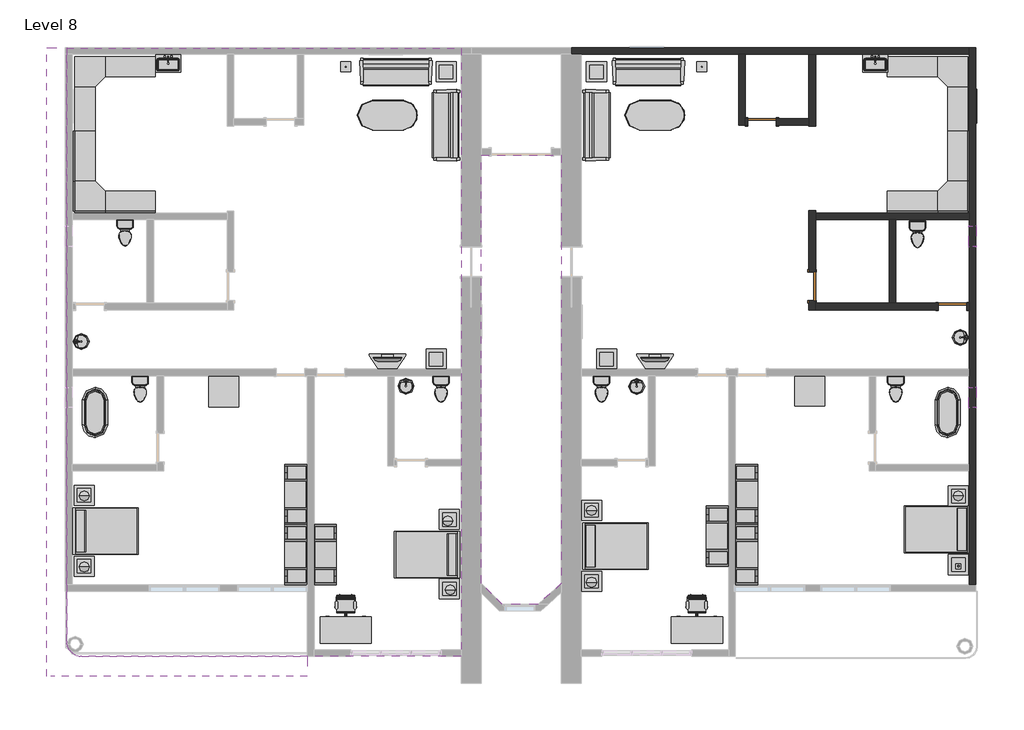
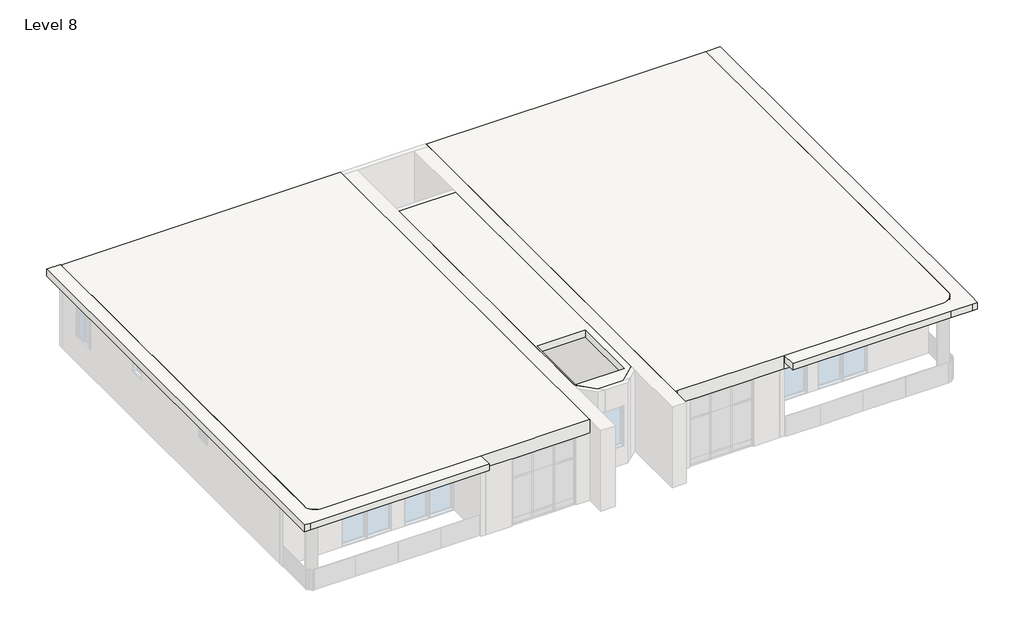
# One storey, part 3 of 3: 42 furniture elements, 14 flow terminals, 10 light fixtures, 9 walls, 3 doors, 3 slabs, 3 windows.
# Revit data of these elements (continued)
# Elements 40, 41 (IfcFurniture, "TV Stand : TV Stand") (continued)
#   Phase Created = New Construction
#   Materials on its faces: "Melamine - Gray", "Glass - Shelves"
# Elements 42, 43, 44, 45, 46, 47, 48, 49, 50, 51, 52, 53 (IfcFurniture, "Table-Coffee : 24\" x 24\" x 24\"")
#   Phase Created = New Construction
#   Materials on its faces: "Glass - Clear, Grey"
# Elements 54, 55 (IfcFurniture, "Table-Dining Oval : 36\" x 72\"")
#   Phase Created = New Construction
#   Materials on its faces: "Steel, Chrome Plated", "Glass - Clear, Grey"
# Elements 56, 57 (IfcFurniture, "Table-Rectangular : 36\" x 36\"")
#   Phase Created = New Construction
#   Materials on its faces: "Birch"
# Elements 58, 59 (IfcFurniture, "Work Station Cubicle : 96\" x 96\"")
#   Phase Created = New Construction
#   Materials on its faces: "Textile - Light Gray", "Laminate, Ivory, Matte"
# Element 60 (IfcLightFixture, "100W - 120V")
#   Mark = "94"
#   Phase Created = New Construction
#   Materials on its faces: "Steel, Chrome Plated", "Glass, Frosted"
# Element 61 (IfcLightFixture, "100W - 120V")
#   Mark = "95"
#   Phase Created = New Construction
#   Materials on its faces: "Steel, Chrome Plated", "Glass, Frosted"
# Element 62 (IfcLightFixture, "Table Lamp - Hemispheric : 60W - 120V")
#   Mark = "96"
#   Phase Created = New Construction
#   Materials on its faces: "Steel, Chrome Plated", "Glass, Frosted", "Birch"
# Element 63 (IfcLightFixture, "Table Lamp - Hemispheric : 60W - 120V")
#   Mark = "97"
#   Phase Created = New Construction
#   Materials on its faces: "Steel, Chrome Plated", "Glass, Frosted", "Birch"
# Element 64 (IfcLightFixture, "Table Lamp - Hemispheric : 60W - 120V")
#   Mark = "98"
#   Phase Created = New Construction
#   Materials on its faces: "Steel, Chrome Plated", "Glass, Frosted", "Birch"
# Element 65 (IfcLightFixture, "Table Lamp - Hemispheric : 60W - 120V")
#   Mark = "99"
#   Phase Created = New Construction
#   Materials on its faces: "Steel, Chrome Plated", "Glass, Frosted", "Birch"
# Element 66 (IfcLightFixture, "Table Lamp - Hemispheric : 60W - 120V")
#   Mark = "100"
#   Phase Created = New Construction
#   Materials on its faces: "Steel, Chrome Plated", "Glass, Frosted", "Birch"
# Element 67 (IfcLightFixture, "Table Lamp - Hemispheric : 60W - 120V")
#   Mark = "101"
#   Phase Created = New Construction
#   Materials on its faces: "Steel, Chrome Plated", "Glass, Frosted", "Birch"
# Element 68 (IfcLightFixture, "Table Lamp - Hemispheric : 60W - 120V")
#   Mark = "102"
#   Phase Created = New Construction
#   Materials on its faces: "Steel, Chrome Plated", "Glass, Frosted", "Birch"
# Element 69 (IfcLightFixture, "Table Lamp - Hemispheric : 60W - 120V")
#   Mark = "103"
#   Phase Created = New Construction
#   Materials on its faces: "Steel, Chrome Plated", "Glass, Frosted", "Birch"
# Element 70 (IfcSlab, "Generic - 12\" cream")
#   Height Offset From Level = 12' - 0"
#   Phase Created = New Construction
#   Materials on its faces: "Parking Stripe"
# Element 71 (IfcSlab, "Generic - 12\" white")
#   built-in parameter 1001955 = 3.14159 (stored number, unit not read)
#   Height Offset From Level = 12' - 0"
#   Phase Created = New Construction
#   Materials on its faces: "Door - Frame"
# Element 72 (IfcSlab, "Generic - 12\" white")
#   Height Offset From Level = 12' - 0"
#   Phase Created = New Construction
#   Materials on its faces: "Door - Frame"
# Elements 73, 74, 75, 76, 77, 78, 79, 80 (IfcWall, "Generic - 8\" cream")
#   Top Offset = 0' - 0"
#   Base Offset = 0' - 0"
#   Unconnected Height = 10' - 0"
#   wall height = 10' - 0"
#   Phase Created = New Construction
#   Base Constraint = Level 8
#   Materials on its faces: "Parking Stripe"
# Element 81 (IfcWall, "Generic - 8\" white")
#   Top Offset = 0' - 0"
#   Base Offset = 0' - 0"
#   Unconnected Height = 10' - 0"
#   wall height = 10' - 0"
#   Phase Created = New Construction
#   Base Constraint = Level 8
#   Materials on its faces: "Door - Frame", "Parking Stripe"
# Element 82 (IfcWindow, "Louvers with Trim : 24\" x 24\"")
#   Mark = "186"
#   Phase Created = New Construction
#   Materials on its faces: "Glass", "Iron, Ductile"
# Element 83 (IfcWindow, "Louvers with Trim : 24\" x 24\"")
#   Mark = "187"
#   Phase Created = New Construction
#   Materials on its faces: "Glass", "Iron, Ductile"
# Element 84 (IfcWindow, "Slider with Trim : 36\" x 48\"")
#   Mark = "183"
#   Phase Created = New Construction
#   Materials on its faces: "Iron, Ductile", "Glass"
# Materials
#   "Wood - Birch - Solid Stained Light Low Gloss": class "Wood", colour RGB 210 159 95, transparency 0, Cost = 0
#   "Paint - Sienna": colour RGB 118 70 51, transparency 0, Cost = 0
#   "Steel, Polished": class "Metal", colour RGB 57 57 57, transparency 0, Description = "Polished steel", Cost = 0
#   "Porcelain, Linen": class "Ceramic", colour RGB 249 239 230, transparency 0, Description = "Porcelain, linen", Cost = 0
#   "Laminate, Linen, Matte": class "Plastic", colour RGB 249 239 230, transparency 0, Description = "Plastic Laminate - Linen, Matte", Cost = 0
#   "Porcelain, Ivory": class "Ceramic", colour RGB 247 247 239, transparency 0, Description = "Porcelain, ivory", Cost = 0
#   "Laminate, Ivory, Matte": class "Plastic", colour RGB 247 247 239, transparency 0, Description = "Plastic Laminate - Ivory, Matte", Cost = 0
#   "Birch": class "Wood", colour RGB 224 178 126, transparency 0, Description = "Betula Alleghaniensis", Cost = 0
#   "Linen, White": class "Textile", colour RGB 247 247 239, transparency 0, Description = "Linen, white", Cost = 0
#   "Plastic, Opaque Black": class "Plastic", colour RGB 0 0 0, transparency 0.7, Description = "Plastic, generic, opaque black", Cost = 0
#   "Textile - Slate Blue": class "Fabric", colour RGB 98 102 118, transparency 0
#   "Steel, Chrome Plated": class "Metal", colour RGB 17 17 17, transparency 0, Description = "Chromiuim plated steel", Cost = 0
#   "Cherry": class "Wood", colour RGB 226 177 128, transparency 0, Description = "Prunus Serotina", Cost = 0
#   "Linen, Beige": class "Textile", colour RGB 249 239 230, transparency 0, Description = "Linen, beige", Cost = 0
#   "Melamine - Gray": class "Wood", colour RGB 49 49 49, transparency 0
#   "Glass - Clear, Grey": class "Glass", colour RGB 252 255 255, transparency 0.64
#   "Textile - Light Gray": class "Fabric", colour RGB 204 204 204, transparency 0
#   "Glass, Frosted": class "Glass", colour RGB 250 244 225, transparency 0.55, Description = "physical material", Cost = 0
#   "Parking Stripe": class "Paint", colour RGB 250 250 91, transparency 0, Cost = 0
#   "Door - Frame": colour RGB 118 70 51, transparency 0, Cost = 0
#   "Iron, Ductile": class "Metal", colour RGB 0 0 0, transparency 0, Description = "Ductile cast iron", Cost = 0
#   "Glass": class "Glass", colour RGB 0 128 192, transparency 0.75, Description = "Soda Lime Glass", Cost = 0
#   "TV - Black": colour RGB 49 49 49, transparency 0
#   "TV - Glass": colour RGB 157 157 157, transparency 0.9
#   "TV - Screen": colour RGB 0 0 0, transparency 0
#   "Glass - Shelves": class "Glass", colour RGB 167 167 167, transparency 0.9
